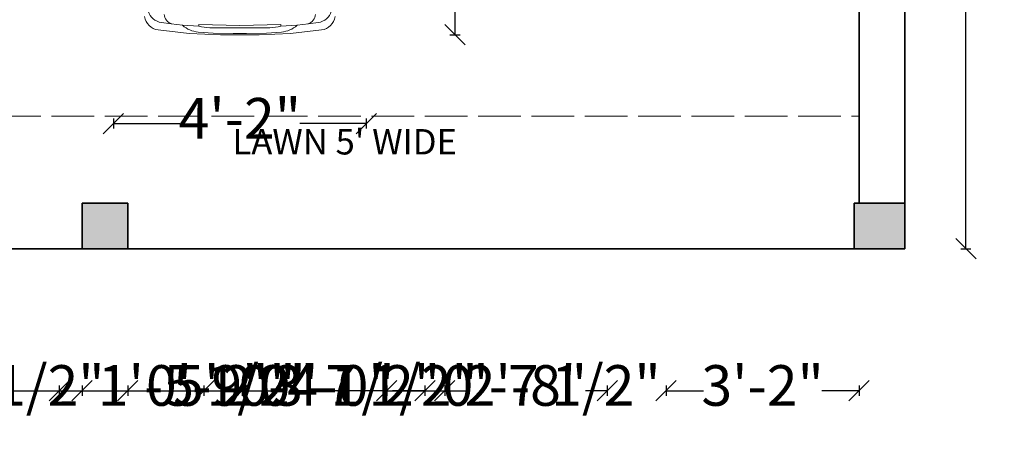
# Model space of a CAD drawing. Units: inches. Extents: x 2558 to 3026, y 433 to 1053.
# Tile 2 of 8: x 2795 to 2989, y 433 to 518. Entities that reach past the tile are written whole.
import ezdxf

# ---------------------------------------------------------------- set-up
doc = ezdxf.new("R2010")
doc.units = ezdxf.units.IN
doc.linetypes.add('ACAD_ISO02W100', pattern=[15, 12, -3])
for name, color, linetype, lineweight in [('0_Equip', 250, 'Continuous', 13), ('A-ANNO-DIMS', 2, 'Continuous', 18), ('A-AREA-IDEN', 7, 'Continuous', 18), ('A-COLS', 7, 'Continuous', 35), ('A-COLS-PATT', 8, 'Continuous', 18), ('A-WALL', 7, 'Continuous', 35), ('L-PLNT-BNDY', 253, 'ACAD_ISO02W100', 18)]:
    doc.layers.add(name, color=color, linetype=linetype, lineweight=lineweight)
doc.styles.get("Standard").update_dxf_attribs({"font": 'arial.ttf'})
doc.dimstyles.new('ISO-25', dxfattribs={"dimtxt": 8, "dimasz": 4, "dimexe": 1, "dimexo": 1, "dimgap": 1, "dimtad": 0, "dimtih": 1, "dimtoh": 1, "dimlunit": 3, "dimtxsty": 'Standard', "dimblk": 'OBLIQUE', "dimcen": 2.5, "dimclrt": 1, "dimadec": 0, "dimazin": 0, "dimtfac": 1, "dimtmove": 0, "dimatfit": 3, "dimfxl": 1, "dimfxlon": 1, "dimarcsym": 0})

# ---------------------------------------------------------------- blocks, each defined once
blk = doc.blocks.new('_Oblique')
at = {"color": 0, "linetype": 'ByBlock', "lineweight": -2}
blk.add_line((-0.5, -0.5), (0.5, 0.5), dxfattribs=at)
blk = doc.blocks.new('*D19')
at = {"layer": 'A-ANNO-DIMS', "color": 0, "lineweight": -2, "transparency": 16777216}
for p, q in [((2980.65, 1012.82), (2982.65, 1012.82)), ((2981.65, 1012.82), (2981.65, 747.89)), ((2981.65, 472.82), (2981.65, 737.76)), ((2980.65, 472.82), (2982.65, 472.82))]:
    blk.add_line(p, q, dxfattribs=at)
at = {"layer": 'Defpoints', "color": 0, "transparency": 16777216}
for p in [(2969.63, 1012.82), (2969.63, 472.82), (2981.65, 472.82)]:
    blk.add_point(p, dxfattribs=at)
at = {"layer": 'A-ANNO-DIMS', "color": 0, "lineweight": -2, "transparency": 16777216, "xscale": 4, "yscale": 4, "zscale": 4}
for p, rotation in [((2981.65, 1012.82), 90), ((2981.65, 472.82), 270)]:
    blk.add_blockref('_Oblique', p, dxfattribs=dict(at, rotation=rotation))
at = {"layer": 'A-ANNO-DIMS', "color": 0, "transparency": 16777216, "insert": (2981.65, 742.82), "char_height": 8, "attachment_point": 5}
blk.add_mtext("45'", dxfattribs=at)
blk = doc.blocks.new('A$C4C7B54D1')
at = {"layer": '0_Equip', "ltscale": 0.1}
for p, q in [((-1.2767, -1.9721), (-1.3526, -1.9616)), ((-0.1746, -1.9721), (-0.0987, -1.9616)), ((-1.3797, -2.0208), (-1.1314, -2.0483)), ((-1.1845, -1.9838), (-1.2767, -1.9721)), ((-1.055, -1.9908), (-1.1845, -1.9838)), ((-1.1314, -2.0483), (-0.8803, -2.0598)), ((-1.0585, -2.0375), (-0.9383, -2.0469)), ((-1.055, -1.9768), (-1.055, -1.9908)), ((-0.7257, -1.985), (-1.055, -1.9768)), ((-0.9663, -2.0048), (-0.7257, -2.0048)), ((-0.9383, -2.0469), (-0.7784, -2.0504)), ((-0.7257, -1.985), (-0.3964, -1.9768)), ((-0.4851, -2.0048), (-0.7257, -2.0048)), ((-0.5131, -2.0469), (-0.673, -2.0504)), ((-0.3199, -2.0483), (-0.5711, -2.0598)), ((-0.3929, -2.0375), (-0.5131, -2.0469)), ((-0.3964, -1.9768), (-0.3964, -1.9908)), ((-0.3964, -1.9908), (-0.2668, -1.9838)), ((-0.0716, -2.0208), (-0.3199, -2.0483)), ((-0.2668, -1.9838), (-0.1746, -1.9721)), ((-0.8803, -2.0598), (-0.7257, -2.0598)), ((-0.7784, -2.0504), (-0.7257, -2.0504)), ((-0.673, -2.0504), (-0.7257, -2.0504)), ((-0.5711, -2.0598), (-0.7257, -2.0598))]:
    blk.add_line(p, q, dxfattribs=at)
for centre, radius, start, end in [((-1.3393, -1.8393), 0.123, 194.49857, 263.78362), ((-0.1121, -1.8393), 0.123, 276.21638, 345.50143), ((-1.3628, -1.8937), 0.1282, 189.09297, 262.41532), ((-1.2452, -1.8915), 0.0853, 183.20552, 252.64053), ((-0.2061, -1.8915), 0.0853, 287.35947, 356.79448), ((-0.0885, -1.8937), 0.1282, 277.58468, 350.90703), ((-1.0413, -1.8225), 0.2157, 228.40601, 265.43909), ((-0.896, -1.272), 0.7362, 257.5275, 264.52088), ((-0.5554, -1.272), 0.7362, 275.47912, 282.4725), ((-0.41, -1.8225), 0.2157, 274.56091, 311.59399)]:
    blk.add_arc(centre, radius, start, end, dxfattribs=at)
blk = doc.blocks.new('*D43')
at = {"layer": 'A-ANNO-DIMS', "color": 0, "lineweight": -2, "transparency": 16777216}
for p, q in [((2880.07, 631.47), (2882.07, 631.47)), ((2881.07, 631.47), (2881.07, 578.35)), ((2881.07, 514.96), (2881.07, 568.08)), ((2880.07, 514.96), (2882.07, 514.96))]:
    blk.add_line(p, q, dxfattribs=at)
at = {"layer": 'Defpoints', "color": 0, "transparency": 16777216}
for p in [(2863.59, 631.47), (2881.07, 631.47), (2863.59, 514.96)]:
    blk.add_point(p, dxfattribs=at)
at = {"layer": 'A-ANNO-DIMS', "color": 0, "lineweight": -2, "transparency": 16777216, "xscale": 4, "yscale": 4, "zscale": 4}
for p, rotation in [((2881.07, 631.47), 90), ((2881.07, 514.96), 270)]:
    blk.add_blockref('_Oblique', p, dxfattribs=dict(at, rotation=rotation))
at = {"layer": 'A-ANNO-DIMS', "color": 1, "transparency": 16777216, "insert": (2881.07, 573.21), "char_height": 8, "attachment_point": 5}
blk.add_mtext('CAR 9\'-8 1/2"', dxfattribs=at)
blk = doc.blocks.new('*D44')
at = {"layer": 'A-ANNO-DIMS', "color": 0, "lineweight": -2, "transparency": 16777216}
for p, q in [((2813.8, 498.48), (2813.8, 496.48)), ((2863.59, 498.48), (2863.59, 496.48)), ((2813.8, 497.48), (2826.9, 497.48)), ((2863.59, 497.48), (2850.49, 497.48))]:
    blk.add_line(p, q, dxfattribs=at)
at = {"layer": 'Defpoints', "color": 0, "transparency": 16777216}
for p in [(2813.8, 514.96), (2863.59, 514.96), (2863.59, 497.48)]:
    blk.add_point(p, dxfattribs=at)
at = {"layer": 'A-ANNO-DIMS', "color": 0, "lineweight": -2, "transparency": 16777216, "xscale": 4, "yscale": 4, "zscale": 4, "rotation": 180}
blk.add_blockref('_Oblique', (2813.8, 497.48), dxfattribs=at)
at = {"layer": 'A-ANNO-DIMS', "color": 0, "lineweight": -2, "transparency": 16777216, "xscale": 4, "yscale": 4, "zscale": 4}
blk.add_blockref('_Oblique', (2863.59, 497.48), dxfattribs=at)
at = {"layer": 'A-ANNO-DIMS', "color": 1, "transparency": 16777216, "insert": (2838.69, 497.48), "char_height": 8, "attachment_point": 5}
blk.add_mtext('4\'-2"', dxfattribs=at)
blk = doc.blocks.new('*D45')
at = {"layer": 'A-ANNO-DIMS', "color": 0, "lineweight": -2, "transparency": 16777216}
for p, q in [((2803.13, 445.87), (2803.13, 443.87)), ((2803.13, 444.87), (2831.63, 444.87)), ((2831.63, 445.87), (2831.63, 443.87)), ((2831.63, 444.87), (2835.63, 444.87))]:
    blk.add_line(p, q, dxfattribs=at)
at = {"layer": 'Defpoints', "color": 0, "transparency": 16777216}
for p in [(2803.13, 799.82), (2831.63, 799.82), (2831.63, 444.87)]:
    blk.add_point(p, dxfattribs=at)
at = {"layer": 'A-ANNO-DIMS', "color": 0, "lineweight": -2, "transparency": 16777216, "xscale": 4, "yscale": 4, "zscale": 4, "rotation": 180}
blk.add_blockref('_Oblique', (2803.13, 444.87), dxfattribs=at)
at = {"layer": 'A-ANNO-DIMS', "color": 0, "lineweight": -2, "transparency": 16777216, "xscale": 4, "yscale": 4, "zscale": 4}
blk.add_blockref('_Oblique', (2831.63, 444.87), dxfattribs=at)
at = {"layer": 'A-ANNO-DIMS', "color": 1, "transparency": 16777216, "insert": (2856.65, 444.87), "char_height": 8, "attachment_point": 5}
blk.add_mtext('2\'-4 1/2"', dxfattribs=at)
blk = doc.blocks.new('*D46')
at = {"layer": 'A-ANNO-DIMS', "color": 0, "lineweight": -2, "transparency": 16777216}
for p, q in [((2922.63, 445.87), (2922.63, 443.87)), ((2922.63, 444.87), (2930, 444.87)), ((2960.63, 444.87), (2953.26, 444.87)), ((2960.63, 445.87), (2960.63, 443.87))]:
    blk.add_line(p, q, dxfattribs=at)
at = {"layer": 'Defpoints', "color": 0, "transparency": 16777216}
for p in [(2922.63, 524.53), (2960.63, 524.53), (2960.63, 444.87)]:
    blk.add_point(p, dxfattribs=at)
at = {"layer": 'A-ANNO-DIMS', "color": 0, "lineweight": -2, "transparency": 16777216, "xscale": 4, "yscale": 4, "zscale": 4, "rotation": 180}
blk.add_blockref('_Oblique', (2922.63, 444.87), dxfattribs=at)
at = {"layer": 'A-ANNO-DIMS', "color": 0, "lineweight": -2, "transparency": 16777216, "xscale": 4, "yscale": 4, "zscale": 4}
blk.add_blockref('_Oblique', (2960.63, 444.87), dxfattribs=at)
at = {"layer": 'A-ANNO-DIMS', "color": 1, "transparency": 16777216, "insert": (2941.63, 444.87), "char_height": 8, "attachment_point": 5}
blk.add_mtext('3\'-2"', dxfattribs=at)
blk = doc.blocks.new('*D49')
at = {"layer": 'A-ANNO-DIMS', "color": 0, "lineweight": -2, "transparency": 16777216}
for p, q in [((2839.13, 445.87), (2839.13, 443.87)), ((2839.13, 444.87), (2845.5, 444.87)), ((2875.13, 444.87), (2868.76, 444.87)), ((2875.13, 445.87), (2875.13, 443.87))]:
    blk.add_line(p, q, dxfattribs=at)
at = {"layer": 'Defpoints', "color": 0, "transparency": 16777216}
for p in [(2839.13, 790.82), (2875.13, 790.82), (2875.13, 444.87)]:
    blk.add_point(p, dxfattribs=at)
at = {"layer": 'A-ANNO-DIMS', "color": 0, "lineweight": -2, "transparency": 16777216, "xscale": 4, "yscale": 4, "zscale": 4, "rotation": 180}
blk.add_blockref('_Oblique', (2839.13, 444.87), dxfattribs=at)
at = {"layer": 'A-ANNO-DIMS', "color": 0, "lineweight": -2, "transparency": 16777216, "xscale": 4, "yscale": 4, "zscale": 4}
blk.add_blockref('_Oblique', (2875.13, 444.87), dxfattribs=at)
at = {"layer": 'A-ANNO-DIMS', "color": 1, "transparency": 16777216, "insert": (2857.13, 444.87), "char_height": 8, "attachment_point": 5}
blk.add_mtext('3\'-0"', dxfattribs=at)
blk = doc.blocks.new('*D50')
at = {"layer": 'A-ANNO-DIMS', "color": 0, "lineweight": -2, "transparency": 16777216}
for p, q in [((2807.63, 445.87), (2807.63, 443.87)), ((2807.63, 444.87), (2826, 444.87)), ((2867.63, 444.87), (2849.27, 444.87)), ((2867.63, 445.87), (2867.63, 443.87))]:
    blk.add_line(p, q, dxfattribs=at)
at = {"layer": 'Defpoints', "color": 0, "transparency": 16777216}
for p in [(2807.63, 649.82), (2867.63, 649.82), (2867.63, 444.87)]:
    blk.add_point(p, dxfattribs=at)
at = {"layer": 'A-ANNO-DIMS', "color": 0, "lineweight": -2, "transparency": 16777216, "xscale": 4, "yscale": 4, "zscale": 4, "rotation": 180}
blk.add_blockref('_Oblique', (2807.63, 444.87), dxfattribs=at)
at = {"layer": 'A-ANNO-DIMS', "color": 0, "lineweight": -2, "transparency": 16777216, "xscale": 4, "yscale": 4, "zscale": 4}
blk.add_blockref('_Oblique', (2867.63, 444.87), dxfattribs=at)
at = {"layer": 'A-ANNO-DIMS', "color": 1, "transparency": 16777216, "insert": (2837.63, 444.87), "char_height": 8, "attachment_point": 5}
blk.add_mtext('5\'-0"', dxfattribs=at)
blk = doc.blocks.new('*D63')
at = {"layer": 'A-ANNO-DIMS', "color": 0, "lineweight": -2, "transparency": 16777216}
for p, q in [((2757.89, 445.87), (2757.89, 443.87)), ((2757.89, 444.87), (2765.63, 444.87)), ((2765.63, 445.87), (2765.63, 443.87)), ((2765.63, 444.87), (2769.63, 444.87))]:
    blk.add_line(p, q, dxfattribs=at)
at = {"layer": 'Defpoints', "color": 0, "transparency": 16777216}
for p in [(2757.89, 943.82), (2765.63, 943.82), (2765.63, 444.87)]:
    blk.add_point(p, dxfattribs=at)
at = {"layer": 'A-ANNO-DIMS', "color": 0, "lineweight": -2, "transparency": 16777216, "xscale": 4, "yscale": 4, "zscale": 4, "rotation": 180}
blk.add_blockref('_Oblique', (2757.89, 444.87), dxfattribs=at)
at = {"layer": 'A-ANNO-DIMS', "color": 0, "lineweight": -2, "transparency": 16777216, "xscale": 4, "yscale": 4, "zscale": 4}
blk.add_blockref('_Oblique', (2765.63, 444.87), dxfattribs=at)
at = {"layer": 'A-ANNO-DIMS', "color": 1, "transparency": 16777216, "insert": (2790.59, 444.87), "char_height": 8, "attachment_point": 5}
blk.add_mtext('0\'-7 1/2"', dxfattribs=at)
blk = doc.blocks.new('*D69')
at = {"layer": 'A-ANNO-DIMS', "color": 0, "lineweight": -2, "transparency": 16777216}
for p, q in [((2790.04, 445.87), (2790.04, 443.87)), ((2790.04, 444.87), (2807.63, 444.87)), ((2807.63, 445.87), (2807.63, 443.87)), ((2807.63, 444.87), (2811.63, 444.87))]:
    blk.add_line(p, q, dxfattribs=at)
at = {"layer": 'Defpoints', "color": 0, "transparency": 16777216}
for p in [(2790.04, 520.82), (2807.63, 520.82), (2807.63, 444.87)]:
    blk.add_point(p, dxfattribs=at)
at = {"layer": 'A-ANNO-DIMS', "color": 0, "lineweight": -2, "transparency": 16777216, "xscale": 4, "yscale": 4, "zscale": 4, "rotation": 180}
blk.add_blockref('_Oblique', (2790.04, 444.87), dxfattribs=at)
at = {"layer": 'A-ANNO-DIMS', "color": 0, "lineweight": -2, "transparency": 16777216, "xscale": 4, "yscale": 4, "zscale": 4}
blk.add_blockref('_Oblique', (2807.63, 444.87), dxfattribs=at)
at = {"layer": 'A-ANNO-DIMS', "color": 1, "transparency": 16777216, "insert": (2832.21, 444.87), "char_height": 8, "attachment_point": 5}
blk.add_mtext('1\'-5 1/2"', dxfattribs=at)
blk = doc.blocks.new('*D73')
at = {"layer": 'A-ANNO-DIMS', "color": 0, "lineweight": -2, "transparency": 16777216}
for p, q in [((2816.63, 1039.77), (2816.63, 1041.77)), ((2959.63, 1039.77), (2959.63, 1041.77)), ((2816.63, 1040.77), (2870.66, 1040.77)), ((2959.63, 1040.77), (2905.6, 1040.77))]:
    blk.add_line(p, q, dxfattribs=at)
at = {"layer": 'Defpoints', "color": 0, "transparency": 16777216}
for p in [(2959.63, 1040.77), (2816.63, 481.83), (2959.63, 481.82)]:
    blk.add_point(p, dxfattribs=at)
at = {"layer": 'A-ANNO-DIMS', "color": 0, "lineweight": -2, "transparency": 16777216, "xscale": 4, "yscale": 4, "zscale": 4, "rotation": 180}
blk.add_blockref('_Oblique', (2816.63, 1040.77), dxfattribs=at)
at = {"layer": 'A-ANNO-DIMS', "color": 0, "lineweight": -2, "transparency": 16777216, "xscale": 4, "yscale": 4, "zscale": 4}
blk.add_blockref('_Oblique', (2959.63, 1040.77), dxfattribs=at)
at = {"layer": 'A-ANNO-DIMS', "color": 1, "transparency": 16777216, "insert": (2888.13, 1040.77), "char_height": 8, "attachment_point": 5}
blk.add_mtext('11\'-11"', dxfattribs=at)
blk = doc.blocks.new('*D74')
at = {"layer": 'A-ANNO-DIMS', "color": 0, "lineweight": -2, "transparency": 16777216}
for p, q in [((2807.63, 445.87), (2807.63, 443.87)), ((2807.63, 444.87), (2816.63, 444.87)), ((2816.63, 445.87), (2816.63, 443.87)), ((2816.63, 444.87), (2820.63, 444.87))]:
    blk.add_line(p, q, dxfattribs=at)
at = {"layer": 'Defpoints', "color": 0, "transparency": 16777216}
for p in [(2807.63, 472.82), (2816.63, 472.82), (2816.63, 444.87)]:
    blk.add_point(p, dxfattribs=at)
at = {"layer": 'A-ANNO-DIMS', "color": 0, "lineweight": -2, "transparency": 16777216, "xscale": 4, "yscale": 4, "zscale": 4, "rotation": 180}
blk.add_blockref('_Oblique', (2807.63, 444.87), dxfattribs=at)
at = {"layer": 'A-ANNO-DIMS', "color": 0, "lineweight": -2, "transparency": 16777216, "xscale": 4, "yscale": 4, "zscale": 4}
blk.add_blockref('_Oblique', (2816.63, 444.87), dxfattribs=at)
at = {"layer": 'A-ANNO-DIMS', "color": 1, "transparency": 16777216, "insert": (2832.27, 444.87), "char_height": 8, "attachment_point": 5}
blk.add_mtext('0\'-9"', dxfattribs=at)
blk = doc.blocks.new('*D75')
at = {"layer": 'A-ANNO-DIMS', "color": 0, "lineweight": -2, "transparency": 16777216}
for p, q in [((2831.63, 445.87), (2831.63, 443.87)), ((2831.63, 444.87), (2839.13, 444.87)), ((2839.13, 445.87), (2839.13, 443.87)), ((2839.13, 444.87), (2843.13, 444.87))]:
    blk.add_line(p, q, dxfattribs=at)
at = {"layer": 'Defpoints', "color": 0, "transparency": 16777216}
for p in [(2831.63, 799.82), (2839.13, 799.82), (2839.13, 444.87)]:
    blk.add_point(p, dxfattribs=at)
at = {"layer": 'A-ANNO-DIMS', "color": 0, "lineweight": -2, "transparency": 16777216, "xscale": 4, "yscale": 4, "zscale": 4, "rotation": 180}
blk.add_blockref('_Oblique', (2831.63, 444.87), dxfattribs=at)
at = {"layer": 'A-ANNO-DIMS', "color": 0, "lineweight": -2, "transparency": 16777216, "xscale": 4, "yscale": 4, "zscale": 4}
blk.add_blockref('_Oblique', (2839.13, 444.87), dxfattribs=at)
at = {"layer": 'A-ANNO-DIMS', "color": 1, "transparency": 16777216, "insert": (2864.09, 444.87), "char_height": 8, "attachment_point": 5}
blk.add_mtext('0\'-7 1/2"', dxfattribs=at)
blk = doc.blocks.new('*D76')
at = {"layer": 'A-ANNO-DIMS', "color": 0, "lineweight": -2, "transparency": 16777216}
for p, q in [((2879.03, 445.87), (2879.03, 443.87)), ((2879.03, 444.87), (2883.32, 444.87)), ((2911.03, 444.87), (2906.73, 444.87)), ((2911.03, 445.87), (2911.03, 443.87))]:
    blk.add_line(p, q, dxfattribs=at)
at = {"layer": 'Defpoints', "color": 0, "transparency": 16777216}
for p in [(2879.03, 943.82), (2911.03, 943.82), (2911.03, 444.87)]:
    blk.add_point(p, dxfattribs=at)
at = {"layer": 'A-ANNO-DIMS', "color": 0, "lineweight": -2, "transparency": 16777216, "xscale": 4, "yscale": 4, "zscale": 4, "rotation": 180}
blk.add_blockref('_Oblique', (2879.03, 444.87), dxfattribs=at)
at = {"layer": 'A-ANNO-DIMS', "color": 0, "lineweight": -2, "transparency": 16777216, "xscale": 4, "yscale": 4, "zscale": 4}
blk.add_blockref('_Oblique', (2911.03, 444.87), dxfattribs=at)
at = {"layer": 'A-ANNO-DIMS', "color": 1, "transparency": 16777216, "insert": (2895.03, 444.87), "char_height": 8, "attachment_point": 5}
blk.add_mtext('2\'-8"', dxfattribs=at)
blk = doc.blocks.new('*D77')
at = {"layer": 'A-ANNO-DIMS', "color": 0, "lineweight": -2, "transparency": 16777216}
for p, q in [((2867.63, 445.87), (2867.63, 443.87)), ((2867.63, 444.87), (2875.13, 444.87)), ((2875.13, 445.87), (2875.13, 443.87)), ((2875.13, 444.87), (2879.13, 444.87))]:
    blk.add_line(p, q, dxfattribs=at)
at = {"layer": 'Defpoints', "color": 0, "transparency": 16777216}
for p in [(2867.63, 658.82), (2875.13, 658.82), (2875.13, 444.87)]:
    blk.add_point(p, dxfattribs=at)
at = {"layer": 'A-ANNO-DIMS', "color": 0, "lineweight": -2, "transparency": 16777216, "xscale": 4, "yscale": 4, "zscale": 4, "rotation": 180}
blk.add_blockref('_Oblique', (2867.63, 444.87), dxfattribs=at)
at = {"layer": 'A-ANNO-DIMS', "color": 0, "lineweight": -2, "transparency": 16777216, "xscale": 4, "yscale": 4, "zscale": 4}
blk.add_blockref('_Oblique', (2875.13, 444.87), dxfattribs=at)
at = {"layer": 'A-ANNO-DIMS', "color": 1, "transparency": 16777216, "insert": (2900.09, 444.87), "char_height": 8, "attachment_point": 5}
blk.add_mtext('0\'-7 1/2"', dxfattribs=at)

msp = doc.modelspace()

# ---------------------------------------------------------------- hatches: boundary and pattern name
at = {"layer": 'A-COLS-PATT'}
h = msp.add_hatch(color=256, dxfattribs=at)
h.dxf.hatch_style = 1
h.paths.add_polyline_path([(2969.633, 481.825), (2960.633, 481.825), (2959.633, 481.825), (2959.633, 472.825), (2969.633, 472.825)])
h.paths.add_polyline_path([(2816.633, 481.827), (2807.633, 481.827), (2807.633, 472.825), (2816.633, 472.825)])

# ---------------------------------------------------------------- linework, layer by layer
at = {"layer": 'A-COLS'}
for p, q in [((2807.633, 481.827), (2807.633, 472.825)), ((2807.633, 481.827), (2816.633, 481.827)), ((2816.633, 481.827), (2816.633, 472.825)), ((2960.633, 481.825), (2959.633, 481.825)), ((2959.633, 481.825), (2959.633, 472.825)), ((2960.633, 481.825), (2969.633, 481.825))]:
    msp.add_line(p, q, dxfattribs=at)
at = {"layer": 'A-WALL'}
for p, q in [((2969.633, 472.825), (2969.633, 1012.825)), ((2960.633, 481.825), (2960.633, 649.825)), ((2669.633, 472.825), (2969.633, 472.825))]:
    msp.add_line(p, q, dxfattribs=at)
at = {"layer": 'L-PLNT-BNDY', "ltscale": 0.7}
msp.add_line((2738.633, 498.947), (2960.633, 498.947), dxfattribs=at)

# ---------------------------------------------------------------- block references
at = {"layer": '0_Equip', "xscale": 24.59206405529848, "yscale": 24.59206405529848, "zscale": 24.59206405529848}
msp.add_blockref('A$C4C7B54D1', (2856.54, 565.611), dxfattribs=at)

# ---------------------------------------------------------------- texts
at = {"layer": 'A-AREA-IDEN', "insert": (2836.32, 496.392), "char_height": 5, "attachment_point": 1}
msp.add_mtext_dynamic_manual_height_columns("\\pxqc;LAWN 5' WIDE", width=46.06135, gutter_width=12.5, heights=[0], dxfattribs=at)

# ---------------------------------------------------------------- dimensions: what is measured, and where the dimension line sits
at = {"layer": 'A-ANNO-DIMS'}
for base, p1, p2, picture, middle in [((2959.633, 1040.775), (2816.633, 481.827), (2959.633, 481.825), '*D73', (2888.133, 1040.775)), ((2765.633, 444.875), (2757.892, 943.825), (2765.633, 943.825), '*D63', (2790.586, 444.875)), ((2911.025, 444.875), (2879.025, 943.825), (2911.025, 943.825), '*D76', (2895.025, 444.875)), ((2831.633, 444.875), (2803.133, 799.825), (2831.633, 799.825), '*D45', (2856.654, 444.875)), ((2839.133, 444.875), (2831.633, 799.825), (2839.133, 799.825), '*D75', (2864.086, 444.875)), ((2875.133, 444.875), (2839.133, 790.825), (2875.133, 790.825), '*D49', (2857.133, 444.875)), ((2875.133, 444.875), (2867.633, 658.825), (2875.133, 658.825), '*D77', (2900.086, 444.875)), ((2867.633, 444.875), (2807.633, 649.825), (2867.633, 649.825), '*D50', (2837.633, 444.875)), ((2960.633, 444.875), (2922.633, 524.526), (2960.633, 524.526), '*D46', (2941.633, 444.875)), ((2807.633, 444.875), (2790.035, 520.825), (2807.633, 520.825), '*D69', (2832.21, 444.875)), ((2863.592, 497.479), (2813.798, 514.956), (2863.592, 514.956), '*D44', (2838.695, 497.479)), ((2816.633, 444.875), (2807.633, 472.825), (2816.633, 472.825), '*D74', (2832.266, 444.875))]:
    dim = msp.add_linear_dim(base=base, p1=p1, p2=p2, dimstyle='ISO-25', override={"dimdec": 1, "dimlfac": 1, "dimrnd": 0, "dimzin": 1, "dimdsep": 46, "dimlunit": 4, "dimfrac": 2}, dxfattribs=at)
    dim.commit()
    dim.dimension.update_dxf_attribs({"geometry": picture, "text_midpoint": middle})
dim = msp.add_linear_dim(base=(2981.646, 472.825), p1=(2969.633, 1012.825), p2=(2969.633, 472.825), angle=90, dimstyle='ISO-25', override={"dimclrd": 0, "dimclre": 0, "dimclrt": 0}, dxfattribs=at)
dim.commit()
dim.dimension.update_dxf_attribs({"geometry": '*D19', "text_midpoint": (2981.646, 742.825)})
dim = msp.add_linear_dim(base=(2881.069, 631.468), p1=(2863.592, 514.956), p2=(2863.592, 631.468), angle=90, text='CAR <>', dimstyle='ISO-25', override={"dimdec": 1, "dimlfac": 1, "dimrnd": 0, "dimzin": 1, "dimdsep": 46, "dimlunit": 4, "dimfrac": 2}, dxfattribs=at)
dim.commit()
dim.dimension.update_dxf_attribs({"geometry": '*D43', "text_midpoint": (2881.069, 573.212)})

doc.saveas('drawing.dxf')
